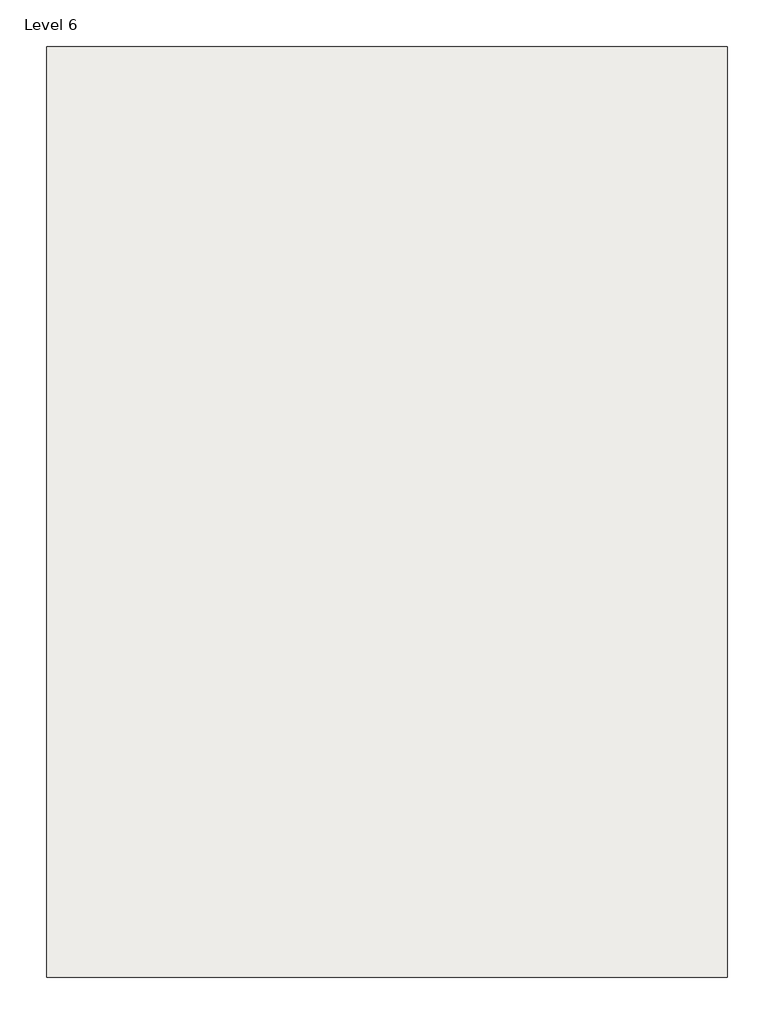
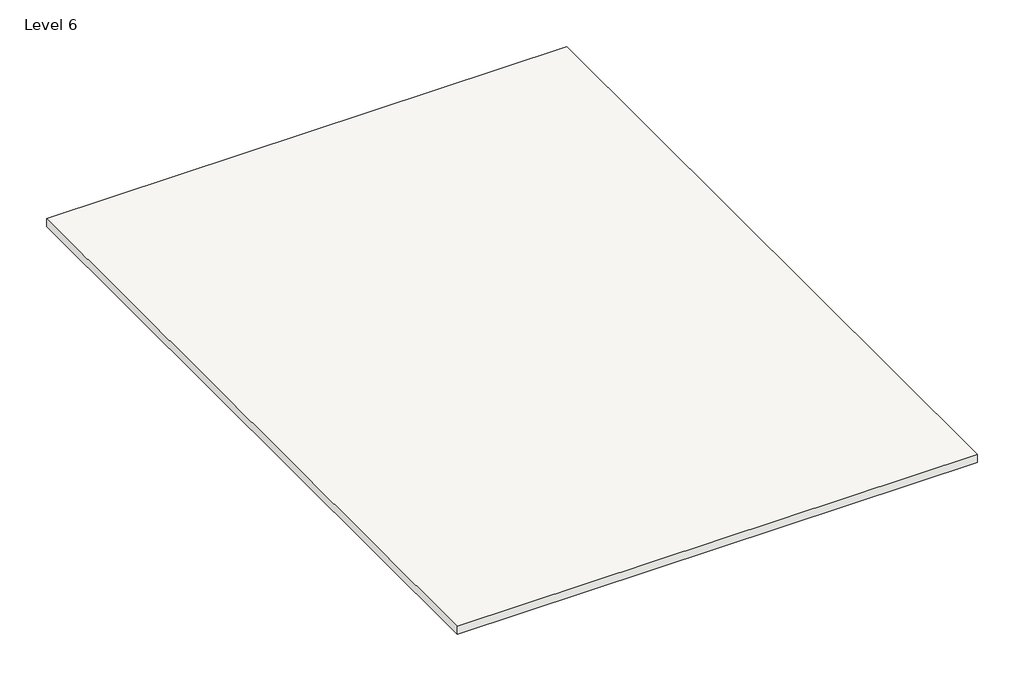
# One storey, incomplete: 1 roof.
"""IFC4 building model written with IfcOpenShell, lengths in millimetres."""

from ifc_helpers import new_model, si_unit, frame, origin, place, context, project, spatial, polyline, outline, extrude, element, save

model = new_model("IFC4")

# Units and contexts
model_context = context("Model", 3, world=origin())
ifc_project = project(units=[si_unit("LENGTHUNIT", "METRE", prefix="MILLI")], contexts=[model_context])

# Site, building, storey
site = spatial("IfcSite", under=ifc_project)
building = spatial("IfcBuilding", under=site)
storey = spatial("IfcBuildingStorey", under=building, Name="Level 6", Elevation=12801.6)

# Roof
placement = place(None, origin())
element("IfcRoof", 1, ObjectType="Generic - 12\"", at=placement, inside=storey, context=model_context, shape_type="SweptSolid", body=[
    extrude(outline(polyline([(-5938.2367314, 6940.7821212), (3421.6632686, 6940.7821212), (3421.6632686, -5860.8178788), (-5938.2367314, -5860.8178788), (-5938.2367314, 6940.7821212)])), frame((0.0, 0.0, 12649.2), z_axis=(0.0, 0.0, 1.0), x_axis=(1.0, 0.0, 0.0)), (0.0, 0.0, 1.0), 152.4),
])

save(model, "model.ifc")

# Revit data of these elements
# Type "Generic - 12\""
#   Assembly Code = "B1020"
#   Layers, outside or top first: 0' - 6" no material (function 1)
# Element 1 (IfcRoof, "Generic - 12\"")
#   built-in parameter 1001705 = 42 (stored number, unit not read)
#   built-in parameter 1001701 = -0.5 (stored number, unit not read)
#   built-in parameter 1001710 = 33615
#   Phase Created = New Construction
#   Materials on its faces: "Default Roof"
# Materials
#   "Default Roof": colour RGB 88 101 114, transparency 0, Cost = 0
